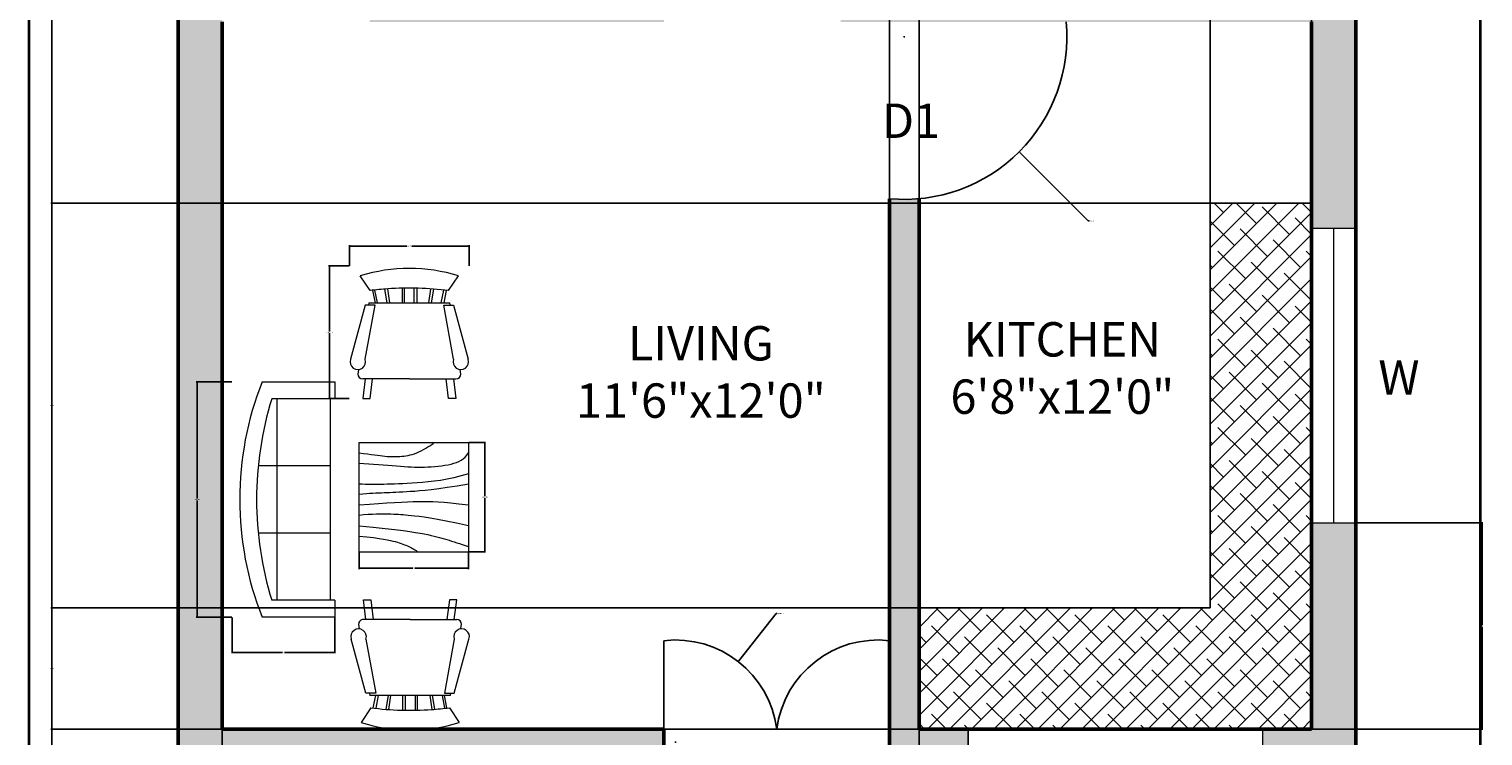
# Model space of a CAD drawing. Units: inches. Extents: x 1972 to 2269, y 1491 to 2023.
# Tile 2 of 3: x 1972 to 2269, y 1687 to 1831. Entities that reach past the tile are written whole.
import ezdxf

# ---------------------------------------------------------------- set-up
doc = ezdxf.new("R2010")
doc.units = ezdxf.units.IN
for name, color, linetype, lineweight in [('A-ANNO-DIMS', 2, 'Continuous', 18), ('A-ANNO-TEXT', 7, 'Continuous', 18), ('A-ANNO-TTLB', 7, 'Continuous', 35), ('A-AREA-IDEN', 7, 'Continuous', 25), ('A-DOOR', 3, 'Continuous', 25), ('A-FLOR-FIXT', 9, 'Continuous', 25), ('A-FURN', 8, 'Continuous', 18), ('A-GLAZ', 4, 'Continuous', 18), ('A-WALL', 7, 'Continuous', 50)]:
    doc.layers.add(name, color=color, linetype=linetype, lineweight=lineweight)
doc.layers.add('A-FLOR-FIXT-PATT', color=251, linetype='Continuous', lineweight=13, true_color=0x636466)
doc.layers.add('A-WALL-PATT', color=18, linetype='Continuous', lineweight=13, true_color=0x000000)
doc.styles.get("Standard").update_dxf_attribs({"font": 'arial.ttf'})
doc.dimstyles.get("Standard").update_dxf_attribs({"dimtxt": 0.18, "dimasz": 0.18, "dimexe": 0.18, "dimexo": 0.0625, "dimgap": 0.09, "dimtad": 0, "dimtih": 1, "dimtoh": 1, "dimdec": 4, "dimzin": 0, "dimdsep": 46, "dimtxsty": 'Standard', "dimcen": 0.09, "dimadec": 0, "dimazin": 0, "dimtfac": 1, "dimtdec": 4, "dimtofl": 0, "dimtmove": 0, "dimatfit": 3, "dimfxl": 1, "dimtolj": 1, "dimtzin": 0, "dimarcsym": 0})

# ---------------------------------------------------------------- blocks, each defined once
blk = doc.blocks.new('Sofa - Roundback 7 ft.')
for p, q in [((-12.00002, -32.4421), (-12.00003, -6.5971)), ((11.99997, -32.4421), (11.99998, -6.5971)), ((-36.000027, -34), (-36.000027, -11.4696)), ((-35.999844, -13.3819), (35.9998, -13.3819)), ((35.99998, -34), (35.99998, -11.4696)), ((-36.000027, -32.4421), (35.99998, -32.4421))]:
    blk.add_line(p, q)
for points in [[(-36.000027, -34), (-42.000027, -34), (-42.000027, -8)], [(41.99998, -8), (41.99998, -34), (35.99998, -34)]]:
    blk.add_lwpolyline(points)
for centre, radius, start, end in [((0, -114.25), 114.25, 68.43141, 111.5686), ((-0.00001, -127.1968), 121.1968, 72.72033, 107.2797)]:
    blk.add_arc(centre, radius, start, end)
blk = doc.blocks.new('Table - Square Woodgrain 42 x 42 in.')
blk.add_line((0, -42), (42, -42))
for points in [[(0, -4), (1.704, -4.2172), (3.2358, -4.4188), (4.615, -4.604), (5.8615, -4.7721), (6.9951, -4.9224), (8.0357, -5.0541), (9.0031, -5.1667), (9.9171, -5.2594), (10.7951, -5.3316), (11.6445, -5.3836), (12.4702, -5.4157), (13.277, -5.4283), (14.0698, -5.4217), (14.8535, -5.3964), (15.6331, -5.3526), (16.4133, -5.2908), (17.1986, -5.2103), (17.9913, -5.1062), (18.793, -4.9727), (19.6056, -4.8038), (20.4307, -4.5937), (21.2701, -4.3365), (22.1256, -4.0262), (22.9989, -3.6571), (23.888, -3.2272), (24.7756, -2.7516), (25.6408, -2.2491), (26.4624, -1.7387), (27.2195, -1.2395), (27.891, -0.7703), (28.456, -0.3501), (28.8934, 0.002)], [(0, -42), (0, 0), (42, 0), (42, -42)], [(0, -8), (1.8203, -8.1001), (3.6741, -8.2149), (5.5411, -8.3408), (7.4011, -8.4741), (9.2339, -8.6112), (11.0193, -8.7484), (12.7371, -8.8821), (14.3671, -9.0086), (15.8954, -9.1246), (17.3337, -9.2278), (18.6997, -9.3159), (20.0116, -9.387), (21.2871, -9.4389), (22.5442, -9.4696), (23.8008, -9.477), (25.0749, -9.459), (26.3791, -9.4137), (27.7049, -9.3403), (29.0383, -9.2382), (30.3655, -9.1068), (31.6728, -8.9455), (32.9461, -8.7535), (34.1717, -8.5304), (35.3358, -8.2756), (36.4268, -7.9863), (37.443, -7.6521), (38.3849, -7.2603), (39.253, -6.7986), (40.048, -6.2542), (40.7705, -5.6147), (41.421, -4.8674), (42, -4)], [(42, -12), (39.1784, -12.8621), (36.4519, -13.5654), (33.8246, -14.1294), (31.3004, -14.5731), (28.8832, -14.9161), (26.577, -15.1775), (24.3858, -15.3768), (22.3136, -15.5332), (20.3622, -15.6632), (18.5254, -15.7718), (16.7947, -15.8612), (15.1618, -15.9338), (13.6183, -15.9916), (12.1558, -16.0369), (10.7659, -16.0718), (9.4403, -16.0987), (8.1703, -16.1191), (6.9461, -16.1325), (5.7577, -16.1377), (4.595, -16.1335), (3.4479, -16.1188), (2.3064, -16.0924), (1.1604, -16.0532), (0, -16)], [(42, -16), (37.6529, -16.7365), (33.8802, -17.329), (30.6179, -17.7961), (27.8015, -18.1561), (25.3668, -18.4275), (23.2497, -18.6288), (21.3859, -18.7785), (19.7111, -18.8949), (18.1693, -18.9939), (16.7375, -19.0795), (15.401, -19.1534), (14.1449, -19.217), (12.9544, -19.2717), (11.8148, -19.3191), (10.7113, -19.3606), (9.6291, -19.3976), (8.5534, -19.4323), (7.47, -19.4689), (6.3643, -19.5122), (5.222, -19.5672), (4.0288, -19.6386), (2.7703, -19.7313), (1.4321, -19.8501), (0, -20)], [(0, -24), (3.9243, -23.6805), (7.4766, -23.4138), (10.6891, -23.1954), (13.5943, -23.0205), (16.2247, -22.8847), (18.6125, -22.7832), (20.7903, -22.7116), (22.7903, -22.6651), (24.6563, -22.642), (26.4764, -22.6507), (28.35, -22.7024), (30.3766, -22.8084), (32.6555, -22.98), (35.2861, -23.2283), (38.3678, -23.5645), (42, -24)], [(42, -32), (37.392, -31.017), (33.4585, -30.2231), (30.1291, -29.5949), (27.3334, -29.109), (25.0009, -28.742), (23.0612, -28.4707), (21.4439, -28.2716), (20.0786, -28.1215), (18.8998, -28.0002), (17.8609, -27.9014), (16.9206, -27.8219), (16.0371, -27.7588), (15.1691, -27.709), (14.2748, -27.6693), (13.3128, -27.6368), (12.2415, -27.6083), (11.0295, -27.5824), (9.6867, -27.5643), (8.233, -27.5608), (6.6884, -27.5787), (5.0728, -27.6248), (3.4062, -27.7058), (1.7086, -27.8286), (0, -28)], [(0, -32), (5.4026, -32.5358), (9.9494, -33.019), (13.7424, -33.4553), (16.8834, -33.8505), (19.4743, -34.2106), (21.6171, -34.5413), (23.4136, -34.8486), (24.9657, -35.1382), (26.3614, -35.4156), (27.6332, -35.6841), (28.7995, -35.9467), (29.8788, -36.2064), (30.8897, -36.4661), (31.8507, -36.7288), (32.7802, -36.9973), (33.6968, -37.2747), (34.6175, -37.5635), (35.5531, -37.8651), (36.5128, -38.1805), (37.506, -38.5108), (38.5421, -38.8568), (39.6302, -39.2197), (40.7797, -39.6004), (42, -40)], [(0, -36), (3.0098, -36.2857), (5.5354, -36.5643), (7.6368, -36.8359), (9.374, -37.1009), (10.807, -37.3597), (11.9957, -37.6126), (13.0002, -37.8599), (13.8804, -38.102), (14.6874, -38.3393), (15.4365, -38.5729), (16.1338, -38.8041), (16.7858, -39.0341), (17.3987, -39.264), (17.9787, -39.4952), (18.5322, -39.7288), (19.0655, -39.9662), (19.5832, -40.2081), (20.0842, -40.4544), (20.5657, -40.7046), (21.0249, -40.9581), (21.459, -41.2144), (21.8653, -41.4731), (22.2409, -41.7335), (22.5831, -41.9951)]]:
    blk.add_lwpolyline(points)
blk = doc.blocks.new('Chair - Rocking')
for p, q in [((-8, -4.5), (-10, -1.5)), ((8, -4.5), (10, -1.5)), ((-7.5, -4.5), (-7, -7)), ((-6.5, -7), (-7.02225, -4.43)), ((-4.5, -7), (-4.96674, -4.19951)), ((-4, -7), (-4.40532, -4.16272)), ((-1.5, -4.05012), (-1.5, -7)), ((-1, -7), (-1, -4.05012)), ((1, -7), (1, -4.04655)), ((1.5, -4.05012), (1.5, -7)), ((4, -7), (4.40187, -4.18694)), ((4.5, -7), (4.96761, -4.19437)), ((6.5, -7), (7, -4.4057)), ((7.5, -4.5), (7, -7)), ((-9, -7.5), (-12, -18.49999)), ((-7, -7.5), (-9, -7.5)), ((-9, -18.49999), (-7, -7.5)), ((-8.23428, -6.99939), (-8.3093, -7.47958)), ((-8.23041, -7), (8.23915, -7)), ((7, -7.5), (9, -7.5)), ((9, -18.49999), (7, -7.5)), ((8.31071, -7.48854), (8.23449, -7.00073)), ((9, -7.5), (12, -18.49999)), ((-10.36644, -20.64523), (-10.5, -21.49999)), ((10.5, -21.49999), (10.3575, -20.58798)), ((-9, -22.49999), (-9.5, -26.49999)), ((0, -22.49999), (-9.5, -22.49999)), ((-8, -26.49999), (-7.5, -22.49999)), ((0, -22.49999), (9.5, -22.49999)), ((8, -26.49999), (7.5, -22.49999)), ((9, -22.49999), (9.5, -26.49999)), ((-9.5, -26.49999), (-8, -26.49999)), ((9.5, -26.49999), (8, -26.49999))]:
    blk.add_line(p, q)
for centre, radius, start, end in [((0, -34.08333), 34.08333, 72.93847, 107.0615), ((0, -68.25004), 64.25, 93.92211, 97.15267), ((0, -68.25004), 64.25, 82.84733, 93.92211), ((-10.5, -18.99999), 1.58114, 161.5651, 18.43495), ((10.5, -18.99999), 1.58114, 161.5651, 18.43495), ((-9.5, -21.49999), 1, 180, 270), ((9.5, -21.49999), 1, 270, 0)]:
    blk.add_arc(centre, radius, start, end)
blk = doc.blocks.new('WINDOW-60IN')
for p, q in [((0, 60), (9, 60)), ((4.5, 60), (4.5, 0)), ((0, 0), (9, 0))]:
    blk.add_line(p, q)
blk = doc.blocks.new('*D22')
at = {"layer": 'A-ANNO-DIMS', "color": 0, "lineweight": -2, "transparency": 16777216}
for p, q in [((2037.67, 1782.9), (2033.5, 1782.9)), ((2033.68, 1782.72), (2033.68, 1769.58)), ((2033.68, 1756.08), (2033.68, 1769.21)), ((2037.67, 1755.9), (2033.5, 1755.9))]:
    blk.add_line(p, q, dxfattribs=at)
at = {"layer": 'A-ANNO-DIMS', "color": 0, "transparency": 16777216}
for points in [[(2033.65, 1782.72), (2033.71, 1782.72), (2033.68, 1782.9)], [(2033.65, 1756.08), (2033.71, 1756.08), (2033.68, 1755.9)]]:
    blk.add_solid(points, dxfattribs=at)
at = {"layer": 'Defpoints', "color": 0, "transparency": 16777216}
for p in [(2033.68, 1782.9), (2037.73, 1782.9), (2037.73, 1755.9)]:
    blk.add_point(p, dxfattribs=at)
at = {"layer": 'A-ANNO-DIMS', "color": 0, "transparency": 16777216, "insert": (2033.68, 1769.4), "char_height": 0.18, "attachment_point": 5}
blk.add_mtext('\\A1;CHAIR 27 TYP.', dxfattribs=at)
blk = doc.blocks.new('*D23')
at = {"layer": 'A-ANNO-DIMS', "color": 0, "lineweight": -2, "transparency": 16777216}
for p, q in [((2037.73, 1782.96), (2037.73, 1787.13)), ((2037.91, 1786.95), (2049.42, 1786.95)), ((2061.99, 1786.95), (2050.48, 1786.95)), ((2062.17, 1782.96), (2062.17, 1787.13))]:
    blk.add_line(p, q, dxfattribs=at)
at = {"layer": 'A-ANNO-DIMS', "color": 0, "transparency": 16777216}
for points in [[(2037.91, 1786.98), (2037.91, 1786.92), (2037.73, 1786.95)], [(2061.99, 1786.98), (2061.99, 1786.92), (2062.17, 1786.95)]]:
    blk.add_solid(points, dxfattribs=at)
at = {"layer": 'Defpoints', "color": 0, "transparency": 16777216}
for p in [(2062.17, 1786.95), (2037.73, 1782.9), (2062.17, 1782.9)]:
    blk.add_point(p, dxfattribs=at)
at = {"layer": 'A-ANNO-DIMS', "color": 0, "transparency": 16777216, "insert": (2049.95, 1786.95), "char_height": 0.18, "attachment_point": 5}
blk.add_mtext('\\A1;24 TYP.', dxfattribs=at)
blk = doc.blocks.new('*D24')
at = {"layer": 'A-ANNO-DIMS', "color": 0, "lineweight": -2, "transparency": 16777216}
for p, q in [((2013.8, 1759.29), (2006.5, 1759.29)), ((2006.68, 1759.11), (2006.68, 1735.53)), ((2006.68, 1711.58), (2006.68, 1735.16)), ((2013.8, 1711.4), (2006.5, 1711.4))]:
    blk.add_line(p, q, dxfattribs=at)
at = {"layer": 'A-ANNO-DIMS', "color": 0, "transparency": 16777216}
for points in [[(2006.65, 1759.11), (2006.71, 1759.11), (2006.68, 1759.29)], [(2006.65, 1711.58), (2006.71, 1711.58), (2006.68, 1711.4)]]:
    blk.add_solid(points, dxfattribs=at)
at = {"layer": 'Defpoints', "color": 0, "transparency": 16777216}
for p in [(2006.68, 1759.29), (2013.86, 1759.29), (2013.86, 1711.4)]:
    blk.add_point(p, dxfattribs=at)
at = {"layer": 'A-ANNO-DIMS', "color": 0, "transparency": 16777216, "insert": (2006.68, 1735.35), "char_height": 0.18, "attachment_point": 5}
blk.add_mtext('\\A1;SOFA 48', dxfattribs=at)
blk = doc.blocks.new('*D25')
at = {"layer": 'A-ANNO-DIMS', "color": 0, "lineweight": -2, "transparency": 16777216}
for p, q in [((2013.86, 1711.34), (2013.86, 1704.04)), ((2034.76, 1711.34), (2034.76, 1704.04)), ((2014.04, 1704.22), (2024.11, 1704.22)), ((2034.58, 1704.22), (2024.51, 1704.22))]:
    blk.add_line(p, q, dxfattribs=at)
at = {"layer": 'A-ANNO-DIMS', "color": 0, "transparency": 16777216}
for points in [[(2014.04, 1704.25), (2014.04, 1704.19), (2013.86, 1704.22)], [(2034.58, 1704.25), (2034.58, 1704.19), (2034.76, 1704.22)]]:
    blk.add_solid(points, dxfattribs=at)
at = {"layer": 'Defpoints', "color": 0, "transparency": 16777216}
for p in [(2013.86, 1711.4), (2034.76, 1711.4), (2013.86, 1704.22)]:
    blk.add_point(p, dxfattribs=at)
at = {"layer": 'A-ANNO-DIMS', "color": 0, "transparency": 16777216, "insert": (2024.31, 1704.22), "char_height": 0.18, "attachment_point": 5}
blk.add_mtext('\\A1;21', dxfattribs=at)
blk = doc.blocks.new('*D26')
at = {"layer": 'A-ANNO-DIMS', "color": 0, "lineweight": -2, "transparency": 16777216}
for p, q in [((2062.04, 1746.96), (2065.5, 1746.96)), ((2065.32, 1746.78), (2065.32, 1736.01)), ((2065.32, 1724.88), (2065.32, 1735.65)), ((2062.04, 1724.7), (2065.5, 1724.7))]:
    blk.add_line(p, q, dxfattribs=at)
at = {"layer": 'A-ANNO-DIMS', "color": 0, "transparency": 16777216}
for points in [[(2065.29, 1746.78), (2065.35, 1746.78), (2065.32, 1746.96)], [(2065.29, 1724.88), (2065.35, 1724.88), (2065.32, 1724.7)]]:
    blk.add_solid(points, dxfattribs=at)
at = {"layer": 'Defpoints', "color": 0, "transparency": 16777216}
for p in [(2061.98, 1746.96), (2065.32, 1746.96), (2061.98, 1724.7)]:
    blk.add_point(p, dxfattribs=at)
at = {"layer": 'A-ANNO-DIMS', "color": 0, "transparency": 16777216, "insert": (2065.32, 1735.83), "char_height": 0.18, "attachment_point": 5}
blk.add_mtext('\\A1;TABLE 22', dxfattribs=at)
blk = doc.blocks.new('*D27')
at = {"layer": 'A-ANNO-DIMS', "color": 0, "lineweight": -2, "transparency": 16777216}
for p, q in [((2039.72, 1724.64), (2039.72, 1721.18)), ((2061.98, 1724.64), (2061.98, 1721.18)), ((2039.9, 1721.36), (2050.63, 1721.36)), ((2061.8, 1721.36), (2051.07, 1721.36))]:
    blk.add_line(p, q, dxfattribs=at)
at = {"layer": 'A-ANNO-DIMS', "color": 0, "transparency": 16777216}
for points in [[(2039.9, 1721.39), (2039.9, 1721.33), (2039.72, 1721.36)], [(2061.8, 1721.39), (2061.8, 1721.33), (2061.98, 1721.36)]]:
    blk.add_solid(points, dxfattribs=at)
at = {"layer": 'Defpoints', "color": 0, "transparency": 16777216}
for p in [(2039.72, 1724.7), (2061.98, 1724.7), (2061.98, 1721.36)]:
    blk.add_point(p, dxfattribs=at)
at = {"layer": 'A-ANNO-DIMS', "color": 0, "transparency": 16777216, "insert": (2050.85, 1721.36), "char_height": 0.18, "attachment_point": 5}
blk.add_mtext('\\A1;22', dxfattribs=at)
blk = doc.blocks.new('*D28')
at = {"layer": 'A-ANNO-DIMS', "color": 0, "lineweight": -2, "transparency": 16777216}
for p, q in [((2002.83, 1996.66), (2002.83, 2022.53)), ((2003.01, 2022.35), (2122.54, 2022.35)), ((2242.65, 2022.35), (2123.12, 2022.35)), ((2242.83, 1790.66), (2242.83, 2022.53))]:
    blk.add_line(p, q, dxfattribs=at)
at = {"layer": 'A-ANNO-DIMS', "color": 0, "transparency": 16777216}
for points in [[(2003.01, 2022.38), (2003.01, 2022.32), (2002.83, 2022.35)], [(2242.65, 2022.38), (2242.65, 2022.32), (2242.83, 2022.35)]]:
    blk.add_solid(points, dxfattribs=at)
at = {"layer": 'Defpoints', "color": 0, "transparency": 16777216}
for p in [(2242.83, 2022.35), (2002.83, 1996.6), (2242.83, 1790.6)]:
    blk.add_point(p, dxfattribs=at)
at = {"layer": 'A-ANNO-DIMS', "color": 0, "transparency": 16777216, "insert": (2122.83, 2022.35), "char_height": 0.18, "attachment_point": 5}
blk.add_mtext('\\A1;240', dxfattribs=at)
blk = doc.blocks.new('*D29')
at = {"layer": 'A-ANNO-DIMS', "color": 0, "lineweight": -2, "transparency": 16777216}
for p, q in [((2002.76, 1996.6), (1976.9, 1996.6)), ((1977.08, 1996.42), (1977.08, 1756.78)), ((1977.08, 1516.78), (1977.08, 1756.42)), ((2002.76, 1516.6), (1976.9, 1516.6))]:
    blk.add_line(p, q, dxfattribs=at)
at = {"layer": 'A-ANNO-DIMS', "color": 0, "transparency": 16777216}
for points in [[(1977.05, 1996.42), (1977.11, 1996.42), (1977.08, 1996.6)], [(1977.05, 1516.78), (1977.11, 1516.78), (1977.08, 1516.6)]]:
    blk.add_solid(points, dxfattribs=at)
at = {"layer": 'Defpoints', "color": 0, "transparency": 16777216}
for p in [(1977.08, 1996.6), (2002.83, 1996.6), (2002.83, 1516.6)]:
    blk.add_point(p, dxfattribs=at)
at = {"layer": 'A-ANNO-DIMS', "color": 0, "transparency": 16777216, "insert": (1977.08, 1756.6), "char_height": 0.18, "attachment_point": 5}
blk.add_mtext('\\A1;480', dxfattribs=at)
blk = doc.blocks.new('*D35')
at = {"layer": 'A-ANNO-DIMS', "color": 0, "lineweight": -2, "transparency": 16777216}
for p, q in [((2242.89, 1730.6), (2268.76, 1730.6)), ((2268.58, 1730.42), (2268.58, 1709.78)), ((2268.58, 1688.78), (2268.58, 1709.42)), ((2233.89, 1688.6), (2268.76, 1688.6))]:
    blk.add_line(p, q, dxfattribs=at)
at = {"layer": 'A-ANNO-DIMS', "color": 0, "transparency": 16777216}
for points in [[(2268.55, 1730.42), (2268.61, 1730.42), (2268.58, 1730.6)], [(2268.55, 1688.78), (2268.61, 1688.78), (2268.58, 1688.6)]]:
    blk.add_solid(points, dxfattribs=at)
at = {"layer": 'Defpoints', "color": 0, "transparency": 16777216}
for p in [(2242.83, 1730.6), (2268.58, 1730.6), (2233.83, 1688.6)]:
    blk.add_point(p, dxfattribs=at)
at = {"layer": 'A-ANNO-DIMS', "color": 0, "transparency": 16777216, "insert": (2268.58, 1709.6), "char_height": 0.18, "attachment_point": 5}
blk.add_mtext('\\A1;42', dxfattribs=at)
blk = doc.blocks.new('*D37')
at = {"layer": 'A-ANNO-DIMS', "color": 0, "lineweight": -2, "transparency": 16777216}
for p, q in [((2153.83, 1688.54), (2153.83, 1490.67)), ((2163.83, 1688.54), (2163.83, 1490.67)), ((2154.01, 1490.85), (2158.62, 1490.85)), ((2163.65, 1490.85), (2159.04, 1490.85))]:
    blk.add_line(p, q, dxfattribs=at)
at = {"layer": 'A-ANNO-DIMS', "color": 0, "transparency": 16777216}
for points in [[(2154.01, 1490.88), (2154.01, 1490.82), (2153.83, 1490.85)], [(2163.65, 1490.88), (2163.65, 1490.82), (2163.83, 1490.85)]]:
    blk.add_solid(points, dxfattribs=at)
at = {"layer": 'Defpoints', "color": 0, "transparency": 16777216}
for p in [(2153.83, 1688.6), (2163.83, 1688.6), (2163.83, 1490.85)]:
    blk.add_point(p, dxfattribs=at)
at = {"layer": 'A-ANNO-DIMS', "color": 0, "transparency": 16777216, "insert": (2158.83, 1490.85), "char_height": 0.18, "attachment_point": 5}
blk.add_mtext('\\A1;10', dxfattribs=at)
blk = doc.blocks.new('*D52')
at = {"layer": 'A-ANNO-DIMS', "color": 0, "lineweight": -2, "transparency": 16777216}
for p, q in [((2213.15, 1795.78), (2213.15, 2022.53)), ((2213.33, 2022.35), (2223.02, 2022.35)), ((2233.65, 2022.35), (2223.96, 2022.35)), ((2233.83, 1795.78), (2233.83, 2022.53))]:
    blk.add_line(p, q, dxfattribs=at)
at = {"layer": 'A-ANNO-DIMS', "color": 0, "transparency": 16777216}
for points in [[(2213.33, 2022.38), (2213.33, 2022.32), (2213.15, 2022.35)], [(2233.65, 2022.38), (2233.65, 2022.32), (2233.83, 2022.35)]]:
    blk.add_solid(points, dxfattribs=at)
at = {"layer": 'Defpoints', "color": 0, "transparency": 16777216}
for p in [(2233.83, 2022.35), (2213.15, 1795.72), (2233.83, 1795.72)]:
    blk.add_point(p, dxfattribs=at)
at = {"layer": 'A-ANNO-DIMS', "color": 0, "transparency": 16777216, "insert": (2223.49, 2022.35), "char_height": 0.18, "attachment_point": 5}
blk.add_mtext('\\A1;20.673', dxfattribs=at)
blk = doc.blocks.new('*D53')
at = {"layer": 'A-ANNO-DIMS', "color": 0, "lineweight": -2, "transparency": 16777216}
for p, q in [((2213.09, 1795.72), (1976.9, 1795.72)), ((1977.08, 1795.54), (1977.08, 1754.67)), ((1977.08, 1713.44), (1977.08, 1754.31)), ((2213.09, 1713.26), (1976.9, 1713.26))]:
    blk.add_line(p, q, dxfattribs=at)
at = {"layer": 'A-ANNO-DIMS', "color": 0, "transparency": 16777216}
for points in [[(1977.05, 1795.54), (1977.11, 1795.54), (1977.08, 1795.72)], [(1977.05, 1713.44), (1977.11, 1713.44), (1977.08, 1713.26)]]:
    blk.add_solid(points, dxfattribs=at)
at = {"layer": 'Defpoints', "color": 0, "transparency": 16777216}
for p in [(1977.08, 1795.72), (2213.15, 1795.72), (2213.15, 1713.26)]:
    blk.add_point(p, dxfattribs=at)
at = {"layer": 'A-ANNO-DIMS', "color": 0, "transparency": 16777216, "insert": (1977.08, 1754.49), "char_height": 0.18, "attachment_point": 5}
blk.add_mtext('\\A1;82.46', dxfattribs=at)
blk = doc.blocks.new('*D54')
at = {"layer": 'A-ANNO-DIMS', "color": 0, "lineweight": -2, "transparency": 16777216}
for p, q in [((2153.76, 1713.26), (1976.9, 1713.26)), ((1977.08, 1713.08), (1977.08, 1701.11)), ((1977.08, 1688.78), (1977.08, 1700.75)), ((2153.76, 1688.6), (1976.9, 1688.6))]:
    blk.add_line(p, q, dxfattribs=at)
at = {"layer": 'A-ANNO-DIMS', "color": 0, "transparency": 16777216}
for points in [[(1977.05, 1713.08), (1977.11, 1713.08), (1977.08, 1713.26)], [(1977.05, 1688.78), (1977.11, 1688.78), (1977.08, 1688.6)]]:
    blk.add_solid(points, dxfattribs=at)
at = {"layer": 'Defpoints', "color": 0, "transparency": 16777216}
for p in [(1977.08, 1713.26), (2153.83, 1713.26), (2153.83, 1688.6)]:
    blk.add_point(p, dxfattribs=at)
at = {"layer": 'A-ANNO-DIMS', "color": 0, "transparency": 16777216, "insert": (1977.08, 1700.93), "char_height": 0.18, "attachment_point": 5}
blk.add_mtext('\\A1;24.66', dxfattribs=at)
blk = doc.blocks.new('*D56')
at = {"layer": 'A-ANNO-DIMS', "color": 0, "lineweight": -2, "transparency": 16777216}
for p, q in [((2011.83, 1832.54), (2011.83, 1490.67)), ((2147.83, 1796.54), (2147.83, 1490.67)), ((2012.01, 1490.85), (2079.55, 1490.85)), ((2147.65, 1490.85), (2080.11, 1490.85))]:
    blk.add_line(p, q, dxfattribs=at)
at = {"layer": 'A-ANNO-DIMS', "color": 0, "transparency": 16777216}
for points in [[(2012.01, 1490.88), (2012.01, 1490.82), (2011.83, 1490.85)], [(2147.65, 1490.88), (2147.65, 1490.82), (2147.83, 1490.85)]]:
    blk.add_solid(points, dxfattribs=at)
at = {"layer": 'Defpoints', "color": 0, "transparency": 16777216}
for p in [(2011.83, 1832.6), (2147.83, 1796.6), (2147.83, 1490.85)]:
    blk.add_point(p, dxfattribs=at)
at = {"layer": 'A-ANNO-DIMS', "color": 0, "transparency": 16777216, "insert": (2079.83, 1490.85), "char_height": 0.18, "attachment_point": 5}
blk.add_mtext('\\A1;136', dxfattribs=at)
blk = doc.blocks.new('*D57')
at = {"layer": 'A-ANNO-DIMS', "color": 0, "lineweight": -2, "transparency": 16777216}
for p, q in [((2147.83, 1796.66), (2147.83, 2022.53)), ((2148.01, 2022.35), (2150.68, 2022.35)), ((2153.65, 2022.35), (2150.98, 2022.35)), ((2153.83, 1796.66), (2153.83, 2022.53))]:
    blk.add_line(p, q, dxfattribs=at)
at = {"layer": 'A-ANNO-DIMS', "color": 0, "transparency": 16777216}
for points in [[(2148.01, 2022.38), (2148.01, 2022.32), (2147.83, 2022.35)], [(2153.65, 2022.38), (2153.65, 2022.32), (2153.83, 2022.35)]]:
    blk.add_solid(points, dxfattribs=at)
at = {"layer": 'Defpoints', "color": 0, "transparency": 16777216}
for p in [(2153.83, 2022.35), (2147.83, 1796.6), (2153.83, 1796.6)]:
    blk.add_point(p, dxfattribs=at)
at = {"layer": 'A-ANNO-DIMS', "color": 0, "transparency": 16777216, "insert": (2150.83, 2022.35), "char_height": 0.18, "attachment_point": 5}
blk.add_mtext('\\A1;6', dxfattribs=at)
blk = doc.blocks.new('*D60')
at = {"layer": 'A-ANNO-DIMS', "color": 0, "lineweight": -2, "transparency": 16777216}
for p, q in [((2150.74, 1829.6), (2150.92, 1829.6)), ((2150.83, 1829.51), (2150.83, 1829.69)), ((2188.32, 1792.11), (2174.38, 1806.04)), ((2188.5, 1792.11), (2188.32, 1792.11))]:
    blk.add_line(p, q, dxfattribs=at)
at = {"layer": 'A-ANNO-DIMS', "color": 0, "transparency": 16777216}
blk.add_solid([(2174.41, 1806.06), (2174.36, 1806.02), (2174.26, 1806.17)], dxfattribs=at)
at = {"layer": 'Defpoints', "color": 0, "transparency": 16777216}
for p in [(2150.83, 1829.6), (2174.26, 1806.17)]:
    blk.add_point(p, dxfattribs=at)
at = {"layer": 'A-ANNO-DIMS', "color": 0, "transparency": 16777216, "insert": (2189.05, 1792.11), "char_height": 0.18, "attachment_point": 5}
blk.add_mtext('\\A1;R33.136', dxfattribs=at)
blk = doc.blocks.new('*D62')
at = {"layer": 'A-ANNO-DIMS', "color": 0, "lineweight": -2, "transparency": 16777216}
for p, q in [((2124.71, 1712.14), (2117.13, 1702.46)), ((2124.89, 1712.14), (2124.71, 1712.14)), ((2104.22, 1685.87), (2104.22, 1686.05)), ((2104.13, 1685.96), (2104.31, 1685.96))]:
    blk.add_line(p, q, dxfattribs=at)
at = {"layer": 'A-ANNO-DIMS', "color": 0, "transparency": 16777216}
blk.add_solid([(2117.11, 1702.48), (2117.16, 1702.44), (2117.02, 1702.32)], dxfattribs=at)
at = {"layer": 'Defpoints', "color": 0, "transparency": 16777216}
for p in [(2117.02, 1702.32), (2104.22, 1685.96)]:
    blk.add_point(p, dxfattribs=at)
at = {"layer": 'A-ANNO-DIMS', "color": 0, "transparency": 16777216, "insert": (2125.63, 1712.14), "char_height": 0.18, "attachment_point": 5}
blk.add_mtext('\\A1;2X R20.778', dxfattribs=at)

msp = doc.modelspace()

# ---------------------------------------------------------------- hatches: boundary and pattern name
at = {"layer": 'A-FLOR-FIXT-PATT'}
h = msp.add_hatch(dxfattribs=at)
h.set_pattern_fill('ANSI38', color=256)
h.paths.add_polyline_path([(2233.8266, 1795.7186), (2213.1538, 1795.7186), (2213.1538, 1713.2582), (2153.8266, 1713.2582), (2153.8266, 1688.5987), (2233.8266, 1688.5987)])
at = {"layer": 'A-WALL-PATT'}
h = msp.add_hatch(color=256, dxfattribs=at)
h.dxf.hatch_style = 1
h.paths.add_polyline_path([(2242.8266, 1996.5987), (2002.8266, 1996.5987), (2002.8266, 1972.5987), (2011.8266, 1972.5987), (2011.8266, 1987.5987), (2092.8266, 1987.5987), (2101.8266, 1987.5987), (2233.8266, 1987.5987), (2233.8266, 1938.5987), (2242.8266, 1938.5987)])
h.paths.add_polyline_path([(2101.8266, 1957.5987, -0.08755883), (2092.8266, 1957.5987), (2092.8266, 1933.5987), (2011.8266, 1933.5987), (2011.8266, 1948.5987), (2002.8266, 1948.5987), (2002.8266, 1896.5987), (2011.8266, 1896.5987), (2011.8266, 1927.5987), (2092.8266, 1927.5987), (2092.8266, 1841.5987), (2041.8266, 1841.5987, -0.08755883), (2041.8266, 1832.5987), (2092.8266, 1832.5987), (2101.8266, 1832.5987), (2101.8266, 1868.5987)])
h.paths.add_polyline_path([(2242.8266, 1890.5987), (2233.8266, 1890.5987), (2233.8266, 1841.5987), (2137.8266, 1841.5987, -0.07106781), (2137.8266, 1832.5987), (2147.8266, 1832.5987), (2183.8266, 1832.5987), (2233.8266, 1832.5987), (2233.8266, 1790.5987), (2242.8266, 1790.5987)])
h.paths.add_polyline_path([(2011.8266, 1832.5987), (2011.8266, 1862.5987), (2011.8266, 1872.5987), (2002.8266, 1872.5987), (2002.8266, 1516.5987), (2022.3266, 1516.5987), (2022.3266, 1525.5987), (2011.8266, 1525.5987), (2011.8266, 1679.5987), (2092.8266, 1679.5987), (2092.8266, 1643.5987), (2092.8266, 1573.5987), (2101.8266, 1573.5987), (2101.8266, 1643.5987), (2101.8266, 1679.5987), (2101.8266, 1688.5987), (2011.8266, 1688.5987)])
h.paths.add_polyline_path([(2140.2493, 1525.5987), (2101.8266, 1525.5987), (2092.8266, 1525.5987), (2082.3266, 1525.5987), (2082.3266, 1516.5987), (2140.2493, 1516.5987)])
h.paths.add_polyline_path([(2242.8266, 1568.0987), (2233.8266, 1568.0987), (2233.8266, 1525.5987), (2233.8266, 1516.5987), (2242.8266, 1516.5987)])
h.paths.add_polyline_path([(2242.8266, 1730.5987), (2233.8266, 1730.5987), (2233.8266, 1688.5987), (2223.8266, 1688.5987), (2223.8266, 1679.5987), (2233.8266, 1679.5987), (2233.8266, 1628.0987), (2242.8266, 1628.0987)])
h.paths.add_polyline_path([(2163.8266, 1688.5987), (2153.8266, 1688.5987), (2153.8266, 1796.5987, -0.04536102), (2147.8266, 1796.5987), (2147.8266, 1688.5987), (2147.8266, 1679.5987), (2153.8266, 1679.5987), (2163.8266, 1679.5987)])

# ---------------------------------------------------------------- linework, layer by layer
at = {"layer": 'A-ANNO-TTLB'}
msp.add_lwpolyline([(1972.4438, 2012.9515), (2268.2203, 2012.9515), (2268.2203, 1493.2355), (1972.4438, 1493.2355)], close=True, dxfattribs=at)
at = {"layer": 'A-DOOR'}
for p, q in [((2101.8266, 1706.5987), (2101.8266, 1688.5987)), ((2147.8266, 1688.5987), (2147.8266, 1706.5987))]:
    msp.add_line(p, q, dxfattribs=at)
for centre, radius, start, end in [((2150.8266, 1829.5987), 33.1361, 264.805571, 5.194429), ((2104.2173, 1685.9591), 20.7776, 7.298619, 96.607296), ((2145.4358, 1685.9591), 20.7776, 83.392704, 172.701381)]:
    msp.add_arc(centre, radius, start, end, dxfattribs=at)
at = {"layer": 'A-FLOR-FIXT'}
for p, q in [((2213.1538, 1795.7186), (2213.1538, 1713.2582)), ((2233.8266, 1795.7186), (2213.1538, 1795.7186)), ((2153.8266, 1713.2582), (2213.1538, 1713.2582))]:
    msp.add_line(p, q, dxfattribs=at)
at = {"layer": 'A-WALL'}
for p, q in [((2002.8266, 1516.5987), (2002.8266, 1996.5987)), ((2242.8266, 1996.5987), (2242.8266, 1516.5987)), ((2011.8266, 1688.5987), (2011.8266, 1832.5987)), ((2233.8266, 1832.5987), (2233.8266, 1688.5987)), ((2147.8266, 1796.5987), (2147.8266, 1688.5987)), ((2153.8266, 1796.5987), (2153.8266, 1688.5987)), ((2101.8266, 1688.5987), (2011.8266, 1688.5987)), ((2101.8266, 1679.5987), (2101.8266, 1688.5987)), ((2147.8266, 1688.5987), (2147.8266, 1679.5987)), ((2153.8266, 1688.5987), (2233.8266, 1688.5987))]:
    msp.add_line(p, q, dxfattribs=at)

# ---------------------------------------------------------------- block references
at = {"layer": 'A-FURN'}
msp.add_blockref('Chair - Rocking', (2049.9504, 1782.3956), dxfattribs=at)
at = {"layer": 'A-FURN', "xscale": 0.5701267150111726, "yscale": 0.5701267150111726, "zscale": 0.5701267150111726, "rotation": 90}
msp.add_blockref('Sofa - Roundback 7 ft.', (2015.3791, 1735.3455), dxfattribs=at)
at = {"layer": 'A-FURN', "xscale": 0.5301134628776305, "yscale": 0.5301134628776305, "zscale": 0.5301134628776305}
msp.add_blockref('Table - Square Woodgrain 42 x 42 in.', (2039.7164, 1746.9625), dxfattribs=at)
at = {"layer": 'A-FURN', "rotation": 180}
msp.add_blockref('Chair - Rocking', (2050.1047, 1688.4263), dxfattribs=at)
at = {"layer": 'A-GLAZ'}
msp.add_blockref('WINDOW-60IN', (2233.827, 1730.599), dxfattribs=at)
at = {"layer": 'A-GLAZ', "rotation": 270.0000000000006}
msp.add_blockref('WINDOW-60IN', (2163.8268, 1688.5983), dxfattribs=at)

# ---------------------------------------------------------------- texts
at = {"layer": 'A-ANNO-TEXT', "char_height": 7, "attachment_point": 1}
for s, width, insert in [('\\pxqc;D1', 10.812609, (2146.7781, 1815.9809)), ('\\pxqc;W', 23.220679, (2240.0281, 1763.6667))]:
    msp.add_mtext_dynamic_manual_height_columns(s, width=width, gutter_width=12.5, heights=[0], dxfattribs=dict(at, insert=insert))
at = {"layer": 'A-AREA-IDEN', "char_height": 7, "attachment_point": 1}
for s, width, insert in [('\\pxqc;{\\fArial|b1|i0|c0|p34;LIVING\\P11\'6"x12\'0"}', 56.127421, (2081.3062, 1770.6606)), ('\\pxqc;{\\fArial|b1|i0|c0|p34;KITCHEN\\P6\'8"x12\'0"}', 48.857017, (2158.6059, 1771.4638))]:
    msp.add_mtext_dynamic_manual_height_columns(s, width=width, gutter_width=12.5, heights=[0], dxfattribs=dict(at, insert=insert))

# ---------------------------------------------------------------- dimensions: what is measured, and where the dimension line sits
at = {"layer": 'A-ANNO-DIMS'}
for base, p1, p2, override, picture, middle in [((2242.8266, 2022.3487), (2002.8266, 1996.5987), (2242.8266, 1790.5987), {"dimdec": 0, "dimlfac": 1, "dimrnd": 0, "dimzin": 0, "dimdsep": 46, "dimlunit": 2}, '*D28', (2122.8266, 2022.3487)), ((2153.8266, 2022.3487), (2147.8266, 1796.5987), (2153.8266, 1796.5987), {"dimdec": 0, "dimlfac": 1, "dimrnd": 0, "dimzin": 0, "dimdsep": 46, "dimlunit": 2}, '*D57', (2150.8266, 2022.3487)), ((2233.8266, 2022.3487), (2213.1538, 1795.7186), (2233.8266, 1795.7186), {"dimdec": 3, "dimlfac": 1, "dimrnd": 0, "dimzin": 0, "dimdsep": 46, "dimlunit": 2}, '*D52', (2223.4902, 2022.3487)), ((2147.8266, 1490.8487), (2011.8266, 1832.5987), (2147.8266, 1796.5987), {"dimdec": 0, "dimlfac": 1, "dimrnd": 0, "dimzin": 0, "dimdsep": 46, "dimlunit": 2}, '*D56', (2079.8266, 1490.8487)), ((2061.9812, 1721.3578), (2039.7164, 1724.6977), (2061.9812, 1724.6977), {"dimdec": 0, "dimlfac": 1, "dimrnd": 0, "dimzin": 0, "dimdsep": 46, "dimlunit": 2}, '*D27', (2050.8488, 1721.3578)), ((2163.8266, 1490.8487), (2153.8266, 1688.5987), (2163.8266, 1688.5987), {"dimdec": 0, "dimlfac": 1, "dimrnd": 0, "dimzin": 0, "dimdsep": 46, "dimlunit": 2}, '*D37', (2158.8266, 1490.8487))]:
    dim = msp.add_linear_dim(base=base, p1=p1, p2=p2, dimstyle='Standard', override=override, dxfattribs=at)
    dim.commit()
    dim.dimension.update_dxf_attribs({"geometry": picture, "text_midpoint": middle})
for base, p1, p2, angle, override, picture, middle in [((1977.0766, 1996.5987), (2002.8266, 1516.5987), (2002.8266, 1996.5987), 90, {"dimdec": 0, "dimlfac": 1, "dimrnd": 0, "dimzin": 0, "dimdsep": 46, "dimlunit": 2}, '*D29', (1977.0766, 1756.5987)), ((1977.0766, 1795.7186), (2213.1538, 1713.2582), (2213.1538, 1795.7186), 90, {"dimdec": 2, "dimlfac": 1, "dimrnd": 0, "dimzin": 0, "dimdsep": 46, "dimlunit": 2}, '*D53', (1977.0766, 1754.4884)), ((2268.5766, 1730.5987), (2233.8266, 1688.5987), (2242.8266, 1730.5987), 90, {"dimdec": 0, "dimlfac": 1, "dimrnd": 0, "dimzin": 0, "dimdsep": 46, "dimlunit": 2}, '*D35', (2268.5766, 1709.5987)), ((1977.0766, 1713.2582), (2153.8266, 1688.5987), (2153.8266, 1713.2582), 90, {"dimdec": 2, "dimlfac": 1, "dimrnd": 0, "dimzin": 0, "dimdsep": 46, "dimlunit": 2}, '*D54', (1977.0766, 1700.9284)), ((2013.8587, 1704.2166), (2034.7634, 1711.4002), (2013.8587, 1711.4002), 180, {"dimdec": 0, "dimlfac": 1, "dimrnd": 0, "dimzin": 0, "dimdsep": 46, "dimlunit": 2}, '*D25', (2024.3111, 1704.2166))]:
    dim = msp.add_linear_dim(base=base, p1=p1, p2=p2, angle=angle, dimstyle='Standard', override=override, dxfattribs=at)
    dim.commit()
    dim.dimension.update_dxf_attribs({"geometry": picture, "text_midpoint": middle})
dim = msp.add_radius_dim(center=(2150.8266, 1829.5987), mpoint=(2174.2572, 1806.1678), dimstyle='Standard', override={"dimdec": 3, "dimlfac": 1, "dimrnd": 0, "dimzin": 0, "dimdsep": 46, "dimlunit": 2}, dxfattribs=at)
dim.commit()
dim.dimension.update_dxf_attribs({"geometry": '*D60', "text_midpoint": (2189.0452, 1792.1093), "dimtype": 164})
dim = msp.add_linear_dim(base=(2062.168, 1786.9456), p1=(2037.7329, 1782.8956), p2=(2062.168, 1782.8956), text='<> TYP.', dimstyle='Standard', override={"dimdec": 0, "dimlfac": 1, "dimrnd": 0, "dimzin": 0, "dimdsep": 46, "dimlunit": 2}, dxfattribs=at)
dim.commit()
dim.dimension.update_dxf_attribs({"geometry": '*D23', "text_midpoint": (2049.9504, 1786.9456)})
for base, p1, p2, text, picture, middle in [((2033.6829, 1782.8956), (2037.7329, 1755.8956), (2037.7329, 1782.8956), 'CHAIR <> TYP.', '*D22', (2033.6829, 1769.3956)), ((2006.6751, 1759.2908), (2013.8587, 1711.4002), (2013.8587, 1759.2908), 'SOFA <>', '*D24', (2006.6751, 1735.3455)), ((2065.3211, 1746.9635), (2061.9812, 1724.6977), (2061.9812, 1746.9635), 'TABLE <>', '*D26', (2065.3211, 1735.8306))]:
    dim = msp.add_linear_dim(base=base, p1=p1, p2=p2, angle=90, text=text, dimstyle='Standard', override={"dimdec": 0, "dimlfac": 1, "dimrnd": 0, "dimzin": 0, "dimdsep": 46, "dimlunit": 2}, dxfattribs=at)
    dim.commit()
    dim.dimension.update_dxf_attribs({"geometry": picture, "text_midpoint": middle})
dim = msp.add_radius_dim(center=(2104.2173, 1685.9591), mpoint=(2117.0227, 1702.3216), text='2X <>', dimstyle='Standard', override={"dimdec": 3, "dimlfac": 1, "dimrnd": 0, "dimzin": 0, "dimdsep": 46, "dimlunit": 2}, dxfattribs=at)
dim.commit()
dim.dimension.update_dxf_attribs({"geometry": '*D62', "text_midpoint": (2125.6308, 1712.1391), "dimtype": 164})

doc.saveas('drawing.dxf')
